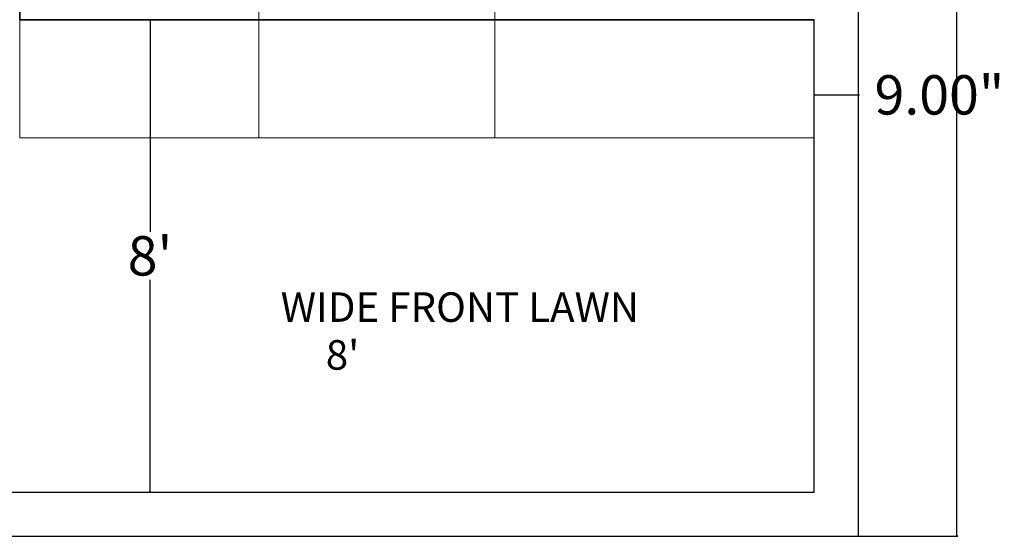
# Model space of a CAD drawing. Units: inches. Extents: x -11 to 443, y 65 to 743.
# Tile 2 of 10: x 162 to 362, y 107 to 212. Entities that reach past the tile are written whole.
import ezdxf

# ---------------------------------------------------------------- set-up
doc = ezdxf.new("R2010")
doc.units = ezdxf.units.IN
doc.header["$MEASUREMENT"] = 0
for name, color, linetype, lineweight in [('A-ANNO-DIMS', 2, 'Continuous', 18), ('A-AREA-IDEN', 2, 'Continuous', 18), ('A-FLOR-EXT', 8, 'Continuous', 18), ('A-GLAZ', 4, 'Continuous', 18), ('A-WALL', 7, 'Continuous', 35), ('A-WALL-SITE', 7, 'Continuous', 30), ('C-PROP', 3, 'Continuous', 30)]:
    doc.layers.add(name, color=color, linetype=linetype, lineweight=lineweight)
doc.styles.get("Standard").update_dxf_attribs({"font": 'italic8.shx'})
doc.dimstyles.get("Standard").update_dxf_attribs({"dimtxt": 8, "dimasz": 0.18, "dimexe": 0.18, "dimexo": 0.0625, "dimgap": 0.09, "dimtad": 0, "dimtih": 1, "dimtoh": 1, "dimzin": 0, "dimdsep": 46, "dimlunit": 3, "dimtxsty": 'Standard', "dimblk": 'CLOSEDBLANK', "dimcen": 0.09, "dimclrd": 6, "dimclre": 5, "dimclrt": 4, "dimadec": 0, "dimazin": 0, "dimtfac": 1, "dimtofl": 0, "dimtmove": 0, "dimatfit": 3, "dimfxl": 1, "dimtolj": 1, "dimtzin": 0, "dimarcsym": 0})

# ---------------------------------------------------------------- blocks, each defined once
blk = doc.blocks.new('_ClosedBlank')
at = {"color": 0, "linetype": 'ByBlock', "lineweight": -2}
for p, q in [((-1, 0.167), (0, 0)), ((-1, 0.167), (-1, -0.167)), ((0, 0), (-1, -0.167))]:
    blk.add_line(p, q, dxfattribs=at)
blk = doc.blocks.new('*D2')
at = {"layer": 'A-ANNO-DIMS', "color": 0, "lineweight": -2, "transparency": 16777216}
for p, q in [((189.03, 211.92), (188.03, 211.92)), ((188.21, 211.74), (188.21, 168.77)), ((188.21, 116.1), (188.21, 159.07)), ((188.27, 115.92), (188.39, 115.92))]:
    blk.add_line(p, q, dxfattribs=at)
at = {"layer": 'Defpoints', "color": 0, "lineweight": 100, "transparency": 16777216}
for p in [(189.09, 211.92), (188.21, 115.92), (188.21, 115.92)]:
    blk.add_point(p, dxfattribs=at)
at = {"layer": 'A-ANNO-DIMS', "color": 0, "lineweight": -2, "transparency": 16777216, "xscale": 0.18, "yscale": 0.18, "zscale": 0.18}
for p, rotation in [((188.21, 211.92), 90), ((188.21, 115.92), 270)]:
    blk.add_blockref('_ClosedBlank', p, dxfattribs=dict(at, rotation=rotation))
at = {"layer": 'A-ANNO-DIMS', "color": 0, "transparency": 16777216, "insert": (188.21, 163.92), "char_height": 8, "attachment_point": 5}
blk.add_mtext("\\A1;8'", dxfattribs=at)
blk = doc.blocks.new('*D6')
at = {"layer": 'A-ANNO-DIMS', "color": 0, "lineweight": -2, "transparency": 16777216}
for p, q in [((332.27, 706.92), (352.4, 706.92)), ((352.22, 706.74), (352.22, 411.77)), ((352.22, 107.1), (352.22, 402.07)), ((332.27, 106.92), (352.4, 106.92))]:
    blk.add_line(p, q, dxfattribs=at)
at = {"layer": 'Defpoints', "color": 0, "lineweight": 100, "transparency": 16777216}
for p in [(332.21, 706.92), (332.21, 106.92), (352.22, 106.92)]:
    blk.add_point(p, dxfattribs=at)
at = {"layer": 'A-ANNO-DIMS', "color": 0, "lineweight": -2, "transparency": 16777216, "xscale": 0.18, "yscale": 0.18, "zscale": 0.18}
for p, rotation in [((352.22, 706.92), 90), ((352.22, 106.92), 270)]:
    blk.add_blockref('_ClosedBlank', p, dxfattribs=dict(at, rotation=rotation))
at = {"layer": 'A-ANNO-DIMS', "color": 0, "transparency": 16777216, "insert": (352.22, 406.92), "char_height": 8, "attachment_point": 5}
blk.add_mtext("\\A1;50'", dxfattribs=at)
blk = doc.blocks.new('*D7')
at = {"layer": 'A-ANNO-DIMS', "color": 0, "lineweight": -2, "transparency": 16777216}
for p, q in [((323.21, 196.7), (323.21, 196.82)), ((323.39, 196.64), (332.03, 196.64)), ((332.21, 196.7), (332.21, 196.82)), ((332.21, 196.64), (332.39, 196.64))]:
    blk.add_line(p, q, dxfattribs=at)
at = {"layer": 'Defpoints', "color": 0, "lineweight": 100, "transparency": 16777216}
for p in [(323.21, 196.64), (332.21, 196.64), (332.21, 196.64)]:
    blk.add_point(p, dxfattribs=at)
at = {"layer": 'A-ANNO-DIMS', "color": 0, "lineweight": -2, "transparency": 16777216, "xscale": 0.18, "yscale": 0.18, "zscale": 0.18, "rotation": 180}
blk.add_blockref('_ClosedBlank', (323.21, 196.64), dxfattribs=at)
at = {"layer": 'A-ANNO-DIMS', "color": 0, "lineweight": -2, "transparency": 16777216, "xscale": 0.18, "yscale": 0.18, "zscale": 0.18}
blk.add_blockref('_ClosedBlank', (332.21, 196.64), dxfattribs=at)
at = {"layer": 'A-ANNO-DIMS', "color": 0, "transparency": 16777216, "insert": (348.67, 196.64), "char_height": 8, "attachment_point": 5}
blk.add_mtext('\\A1;9.00"', dxfattribs=at)
blk = doc.blocks.new('WIN-48x9')
for p, q in [((0, 48), (0, 0)), ((9, 48), (0, 48)), ((3, 0), (3, 48)), ((6, 0), (6, 48)), ((9, 0), (9, 48)), ((0, 0), (9, 0))]:
    blk.add_line(p, q)

msp = doc.modelspace()

# ---------------------------------------------------------------- linework, layer by layer
at = {"layer": 'A-FLOR-EXT'}
for p, q in [((161.709, 211.92), (161.709, 187.92)), ((210.325, 211.92), (210.325, 187.92)), ((258.325, 211.92), (258.325, 187.92)), ((161.709, 187.92), (323.209, 187.92))]:
    msp.add_line(p, q, dxfattribs=at)
at = {"layer": 'A-WALL'}
for q in [(161.709, 227.442), (323.209, 211.92)]:
    msp.add_line((161.709, 211.92), q, dxfattribs=at)
at = {"layer": 'A-WALL-SITE'}
for p, q in [((323.209, 115.92), (323.209, 211.92)), ((53.209, 115.92), (323.209, 115.92))]:
    msp.add_line(p, q, dxfattribs=at)
at = {"layer": 'C-PROP'}
msp.add_lwpolyline([(44.209, 106.92), (332.209, 106.92), (332.209, 706.92), (44.209, 706.92)], close=True, dxfattribs=at)

# ---------------------------------------------------------------- block references
at = {"layer": 'A-GLAZ', "rotation": 89.99999999999991}
msp.add_blockref('WIN-48x9', (258.324, 211.92), dxfattribs=at)

# ---------------------------------------------------------------- texts
at = {"layer": 'A-AREA-IDEN'}
for s, p in [('WIDE FRONT LAWN', (214.762, 150.504)), ("     8'", (214.762, 140.79))]:
    msp.add_text(s, height=6, dxfattribs=at).set_placement(p)

# ---------------------------------------------------------------- dimensions: what is measured, and where the dimension line sits
at = {"layer": 'A-ANNO-DIMS'}
for base, p1, p2, picture, middle in [((352.221, 106.92), (332.209, 706.92), (332.209, 106.92), '*D6', (352.221, 406.92)), ((188.209, 115.92), (189.094, 211.92), (188.209, 115.92), '*D2', (188.209, 163.92))]:
    dim = msp.add_linear_dim(base=base, p1=p1, p2=p2, angle=90, dimstyle='Standard', override={"dimclrd": 0, "dimclre": 0, "dimclrt": 0}, dxfattribs=at)
    dim.commit()
    dim.dimension.update_dxf_attribs({"geometry": picture, "text_midpoint": middle})
dim = msp.add_linear_dim(base=(332.209, 196.639), p1=(323.209, 196.639), p2=(332.209, 196.639), dimstyle='Standard', override={"dimclrd": 0, "dimclre": 0, "dimclrt": 0}, dxfattribs=at)
dim.commit()
dim.dimension.update_dxf_attribs({"geometry": '*D7', "text_midpoint": (348.67, 196.639)})

doc.saveas('drawing.dxf')
